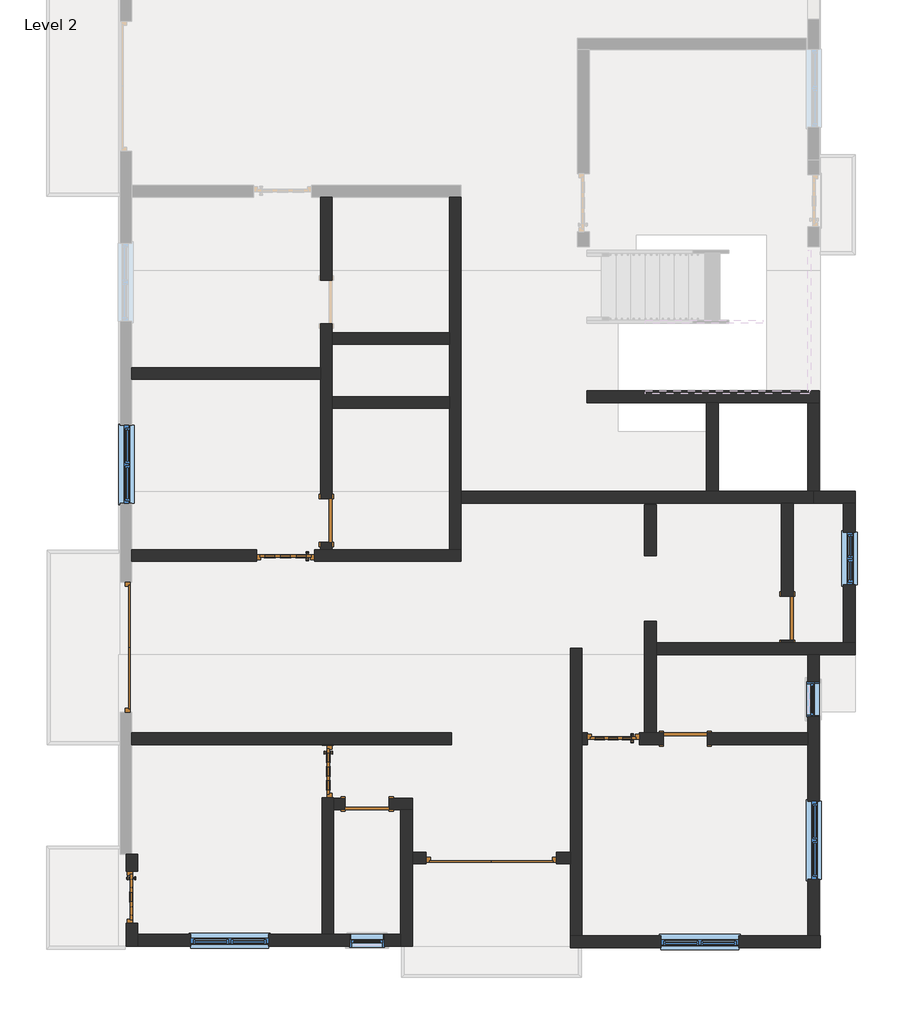
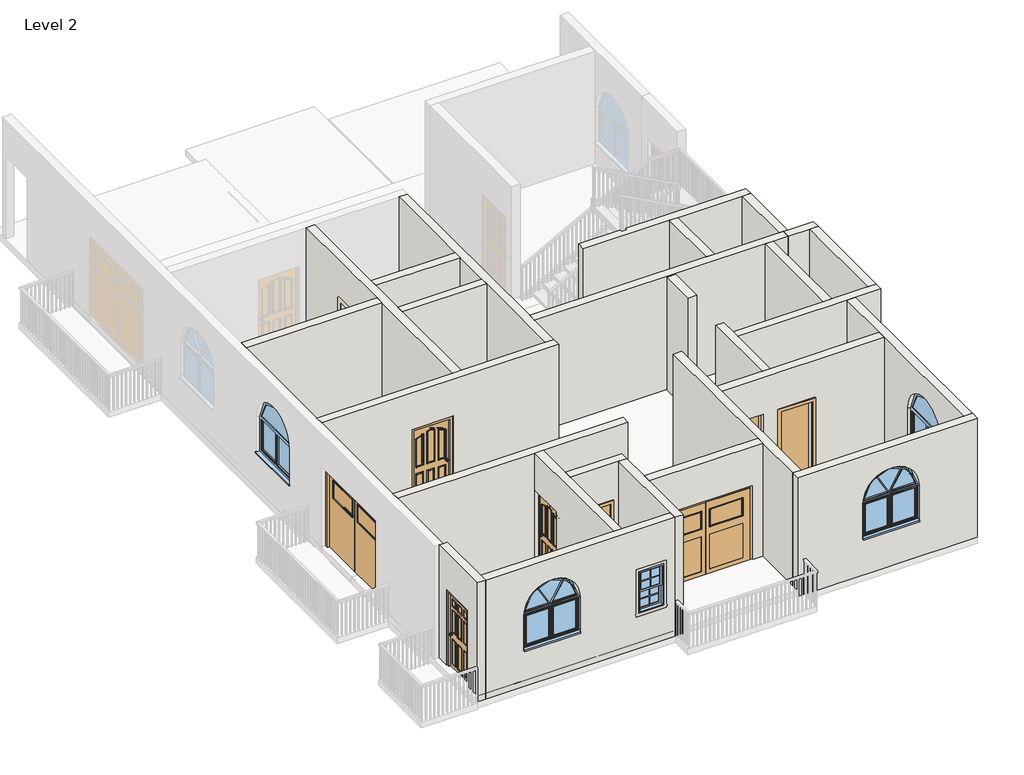
# One storey, part 1 of 7: 27 walls, 10 doors, 7 windows.
# Revit data of these elements (continued)
# Type "Single-Flush : 30\" x 80\"" (continued)
#   Construction Type Id = "MDOOR"
#   Assembly Code = "C1020"
#   Analytic Construction = "Metal"
#   Thickness = 0' - 2"
#   Heat Transfer Coefficient (U) = 0.651978 BTU/(h·ft²·°F)
#   Height = 6' - 8"
#   Trim Projection Ext = 0' - 1"
#   Trim Projection Int = 0' - 1"
#   Trim Width = 0' - 3"
#   Width = 2' - 6"
#   Define Thermal Properties by = 1
#   Define Thermal Properties by = 1
#   Door Material = Door - Panel
#   Frame Material = Door - Frame
#   Visual Light Transmittance = 0
#   Solar Heat Gain Coefficient = 0
#   Function = (empty or 0)
#   Wall Closure = (empty or 0)
# Type "Generic - 9\" w"
#   Assembly Code = "B2010"
#   Layers, outside or top first: 0' - 8" no material (function 1)
# Type "Generic -4.5\" p"
#   Assembly Code = "B2010"
#   Layers, outside or top first: 0' - 8" no material (function 1)
# Type "Window-Double-Hung : 24\" x 42\""
#   Type Mark = "10"
#   Fire Rating = "0.5h"
#   Construction Type Id = "DG-DR"
#   Assembly Code = "B2020100"
#   Analytic Construction = "Double glazing - domestic"
#   Wall Thickness [instance default] = 0' - 6"
#   Window Inset [instance default] = 0' - 0"
#   Visual Light Transmittance = 0.81
#   Thermal Resistance (R) = 1.8146 (h·ft²·°F)/BTU
#   Solar Heat Gain Coefficient = 0.76
#   Muntin Width = 1' - 6"
#   Muntin Height = 1' - 5 1/8"
#   Interior Wall Closure [instance default] = 0' - 1 1/2"
#   Rough Width = 2' - 0 1/2"
#   Rough Height = 3' - 6 1/2"
#   Frame Extension [instance default] = 0' - 1 1/4"
#   Exterior Wall Closure [instance default] = 0' - 0 1/2"
#   Extension Jamb [instance default] = 0' - 1 1/2"
#   Heat Transfer Coefficient (U) = 0.5511 BTU/(h·ft²·°F)
#   Height = 3' - 6"
#   Width = 2' - 0"
#   Define Thermal Properties by = 1
#   Top Muntin Visibility = yes
#   Indicator Visibility [instance default] = yes
#   Extension Jamb Visibility [instance default] = yes
#   Interior Trim Visibility [instance default] = yes
#   Exterior Trim Visibility [instance default] = yes
#   Define Thermal Properties by = 1
#   Bottom Muntin Visibility = yes
#   Muntin Pattern = Muntin Pattern_2x2 : Muntin Pattern_2x2
#   Interior Trim Material = Wood - Stained
#   Interior Trim = Trim-Window-Interior-Flat : Picture Frame
#   Exterior Trim Material = Clad - White
#   Exterior Trim = Trim-Window-Exterior-Flat : with Sill
#   Glass Panel Material = Glass
#   Exterior Frame Material = Clad - White
#   Interior Frame Material = Wood - Stained
#   Wall Closure = (empty or 0)
# Type "Windows_Arched : 1360x910mm"
#   Type Mark = "20"
#   Operation = "UserDefined"
#   Construction Type Id = "GSP4R"
#   Manufacturer = "Revit"
#   Keynote = "L10"
#   Analytic Construction = "1/8 in Pilkington single glazing"
#   Wrap Layers (Ext) from Ext = 0' - 4.03543"
#   Wrap Layers (Int) from Ext = 0' - 6.98819"
#   Window Board Projection = 0' - 0.98425"
#   Window Board Extension = 0' - 0.98425"
#   Visual Light Transmittance = 0.9
#   Solar Heat Gain Coefficient = 0.78
#   Rough Width = 4' - 5.54331"
#   Rough Height = 2' - 11.82677"
#   Height = 2' - 11.82677"
#   Width = 4' - 5.54331"
#   Heat Transfer Coefficient (U) = 0.6496 BTU/(h·ft²·°F)
#   Glazing Thickness = 0' - 0.94488"
#   FrameOffset - External = 0' - 1.9685"
#   Frame Depth = 0' - 2.67717"
#   Default Head Height = 6' - 11.07087"
#   Cill Depth = 0' - 3.44488"
#   Cavity Closer Width = 0' - 1.9685"
#   Cavity Closer Offset from Ext = 0' - 4.03543"
#   Cavity Closer Depth = 0' - 3.34646"
#   Vis - Cavity Closers = yes
#   Define Thermal Properties by = 1
#   Material Trim = Window Frame
#   Material Glass = Glass
#   Material Frame = Window Frame
#   Wall Closure = (empty or 0)
# Type "Windows_Dbl_w-Glazing_Bars : 910x910mm"
#   Type Mark = "33"
#   Operation = "DoublePanelVertical"
#   Construction Type Id = "GSP4R"
#   Manufacturer = "Revit"
#   Keynote = "L10"
#   Analytic Construction = "1/8 in Pilkington single glazing"
#   Wrap Layers (Ext) from Ext = 0' - 4.03543"
#   Wrap Layers (Int) from Ext = 0' - 6.98819"
#   Window Board Projection = 0' - 0.98425"
#   Window Board Extension = 0' - 0.98425"
#   Visual Light Transmittance = 0.9
#   Solar Heat Gain Coefficient = 0.78
#   Rough Width = 2' - 11.82677"
#   Rough Height = 2' - 11.82677"
#   Height = 2' - 11.82677"
#   Width = 2' - 11.82677"
#   Heat Transfer Coefficient (U) = 0.6496 BTU/(h·ft²·°F)
#   Glazing Thickness = 0' - 0.94488"
#   Glazing Bar Thickness = 0' - 0.7874"
#   FrameOffset - External = 0' - 1.9685"
#   Frame Depth = 0' - 2.55906"
#   Default Head Height = 6' - 10.67717"
#   Cill Depth = 0' - 3.44488"
#   Cavity Closer Width = 0' - 1.9685"
#   Cavity Closer Offset from Ext = 0' - 4.03543"
#   Cavity Closer Depth = 0' - 3.34646"
#   Vis - Glazing Bars = yes
#   Vis - Cavity Closers = yes
#   Define Thermal Properties by = 1
#   Material Trim = Window Frame
#   Material Glazing Bars = Window Frame
#   Material Glass = Glass
#   Material Frame = Window Frame
#   Wall Closure = (empty or 0)
# Element 1 (IfcDoor, "Doors_ExtSgl_5 : 910x2110mm")
#   Phase Created = New Construction
#   Materials on its faces: "Door - Panel", "Door - Handle", "Door - Frame/Mullion", "Door - Glazing"
# Element 2 (IfcDoor, "Doors_ExtSgl_6 : 1010x2110mm")
#   Phase Created = New Construction
#   Materials on its faces: "Door - Panel", "Door - Handle", "Door - Frame/Mullion", "Door - Glazing"
# Elements 3, 4 (IfcDoor, "Doors_ExtSgl_6 : 910x2110mm")
#   Phase Created = New Construction
#   Materials on its faces: "Door - Panel", "Door - Handle", "Door - Frame/Mullion", "Door - Glazing"
# Element 5 (IfcDoor, "Doors_Garage_Timber_Side_Hung_Glazing : 2270x2050mm")
#   Phase Created = New Construction
#   Materials on its faces: "Door - Panel", "Door - Frame/Mullion", "Door - Glazing"
# Element 6 (IfcDoor, "Doors_Garage_Timber_Side_Hung_Glazing : 2270x2200mm")
#   Phase Created = New Construction
#   Materials on its faces: "Door - Panel", "Door - Frame/Mullion", "Door - Glazing"
# Elements 7, 8, 9, 10 (IfcDoor, "Single-Flush : 30\" x 80\"")
#   Phase Created = New Construction
#   Materials on its faces: "Door - Frame", "Door - Panel"
# Element 11 (IfcWall, "Generic - 9\" w")
#   Top Offset = 0' - 0"
#   Base Offset = 0' - 0"
#   wall height = 10' - 0"
#   Phase Created = New Construction
#   Base Constraint = Level 2
#   Top Constraint = Level 3
#   Materials on its faces: "Default Wall", "Door - Frame", "Earth"
# Elements 12, 13 (IfcWall, "Generic - 9\" w")
#   Top Offset = 0' - 0"
#   Base Offset = 0' - 0"
#   wall height = 10' - 0"
#   Phase Created = New Construction
#   Base Constraint = Level 2
#   Top Constraint = Level 3
#   Materials on its faces: "Default Wall"
# Element 14 (IfcWall, "Generic - 9\" w")
#   Top Offset = 0' - 0"
#   Base Offset = 0' - 0"
#   wall height = 10' - 0"
#   Phase Created = New Construction
#   Base Constraint = Level 2
#   Top Constraint = Level 3
#   Materials on its faces: "Default Wall", "Door - Frame/Mullion", "Earth"
# Element 15 (IfcWall, "Generic - 9\" w")
#   Top Offset = 0' - 0"
#   Base Offset = 0' - 0"
#   wall height = 10' - 0"
#   Phase Created = New Construction
#   Base Constraint = Level 2
#   Top Constraint = Level 3
#   Materials on its faces: "Default Wall", "Concrete, Lightweight", "Wood - Stained"
# Element 16 (IfcWall, "Generic - 9\" w")
#   Top Offset = 0' - 0"
#   Base Offset = 0' - 0"
#   wall height = 10' - 0"
#   Phase Created = New Construction
#   Base Constraint = Level 2
#   Top Constraint = Level 3
#   Materials on its faces: "Default Wall", "Wood - Stained"
# Element 17 (IfcWall, "Generic - 9\" w")
#   Top Offset = 0' - 0"
#   Base Offset = 0' - 0"
#   wall height = 10' - 0"
#   Phase Created = New Construction
#   Base Constraint = Level 2
#   Top Constraint = Level 3
#   Materials on its faces: "Default Wall", "Earth"
# Elements 18, 19 (IfcWall, "Generic - 9\" w")
#   Top Offset = 0' - 0"
#   Base Offset = 0' - 0"
#   wall height = 10' - 0"
#   Phase Created = New Construction
#   Base Constraint = Level 2
#   Top Constraint = Level 3
#   Materials on its faces: "Default Wall", "Concrete, Lightweight"
# Elements 20, 21, 22, 23, 24, 25, 26, 27, 28, 31, 32, 33, 36, 37 (IfcWall, "Generic -4.5\" p")
#   Top Offset = 0' - 0"
#   Base Offset = 0' - 0"
#   wall height = 10' - 0"
#   Phase Created = New Construction
#   Base Constraint = Level 2
#   Top Constraint = Level 3
#   Materials on its faces: "Default Wall"
# Element 29 (IfcWall, "Generic -4.5\" p")
#   Top Offset = 0' - 0"
#   Base Offset = 0' - 0"
#   wall height = 10' - 0"
#   Phase Created = New Construction
#   Base Constraint = Level 2
#   Top Constraint = Level 3
#   Materials on its faces: "Default Wall", "Concrete, Lightweight"
# Element 30 (IfcWall, "Generic -4.5\" p")
#   Top Offset = 0' - 0"
#   Base Offset = 0' - 0"
#   wall height = 10' - 0"
#   Phase Created = New Construction
#   Base Constraint = Level 2
#   Top Constraint = Level 3
#   Materials on its faces: "Default Wall", "Door - Frame/Mullion"
# Elements 34, 35 (IfcWall, "Generic -4.5\" p")
#   Top Offset = 0' - 0"
#   Base Offset = 0' - 0"
#   wall height = 10' - 0"
#   Phase Created = New Construction
#   Base Constraint = Level 2
#   Top Constraint = Level 3
#   Materials on its faces: "Default Wall", "Earth"
# Element 38 (IfcWindow, "Window-Double-Hung : 24\" x 42\"")
#   Mark = "25"
#   Window Inset = 0' - 0"
#   Interior Wall Closure = 0' - 1 1/2"
#   Frame Extension = 0' - 1 1/4"
#   Exterior Wall Closure = 0' - 0 1/2"
#   Interior Trim Visibility = yes
#   Indicator Visibility = yes
#   Exterior Trim Visibility = yes
#   Phase Created = New Construction
#   Materials on its faces: "Wood - Stained", "Glass", "Clad - White"
# Element 39 (IfcWindow, "Window-Double-Hung : 24\" x 42\"")
#   Mark = "88"
#   Window Inset = 0' - 0"
#   Interior Wall Closure = 0' - 1 1/2"
#   Frame Extension = 0' - 1 1/4"
#   Exterior Wall Closure = 0' - 0 1/2"
#   Interior Trim Visibility = yes
#   Indicator Visibility = yes
#   Exterior Trim Visibility = yes
#   Phase Created = New Construction
#   Materials on its faces: "Wood - Stained", "Glass", "Clad - White"
# Element 40 (IfcWindow, "Windows_Arched : 1360x910mm")
#   Mark = "21"
#   Phase Created = New Construction
#   Materials on its faces: "Window Frame", "Glass"
# Element 41 (IfcWindow, "Windows_Arched : 1360x910mm")
#   Mark = "22"
#   Phase Created = New Construction
#   Materials on its faces: "Window Frame", "Glass"
# Element 42 (IfcWindow, "Windows_Arched : 1360x910mm")
#   Mark = "23"
#   Phase Created = New Construction
#   Materials on its faces: "Window Frame", "Glass"
# Element 43 (IfcWindow, "Windows_Arched : 1360x910mm")
#   Mark = "83"
#   Phase Created = New Construction
#   Materials on its faces: "Window Frame", "Glass"
# Element 44 (IfcWindow, "Windows_Dbl_w-Glazing_Bars : 910x910mm")
#   Mark = "26"
#   Phase Created = New Construction
#   Materials on its faces: "Window Frame", "Glass"
# Materials
#   "Door - Glazing": colour RGB 0 0 255, transparency 0.75
#   "Door - Panel": class "Wood", colour RGB 210 159 95, transparency 0, Cost = 0
#   "Door - Frame/Mullion": class "Wood", colour RGB 212 179 113, transparency 0
#   "Door - Handle": colour RGB 0 0 0, transparency 0
#   "Door - Frame": colour RGB 118 70 51, transparency 0, Cost = 0
#   "Wood - Stained": class "Wood", colour RGB 224 178 126, transparency 0, Cost = 0
#   "Clad - White": class "Wood", colour RGB 242 242 238, transparency 0, Cost = 0
#   "Glass": class "Glass", colour RGB 0 128 192, transparency 0.75, Description = "Soda Lime Glass", Cost = 0
#   "Window Frame": colour RGB 249 249 249, transparency 0
#   "Default Wall": colour RGB 128 128 128, transparency 0, Cost = 0
#   "Earth": class "Generic", colour RGB 97 75 62, transparency 0, Description = "Soil", Cost = 0
#   "Concrete, Lightweight": class "Concrete", colour RGB 142 141 140, transparency 0, Description = "Lightweight concrete", Cost = 0
